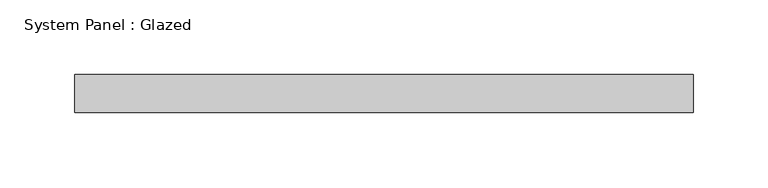
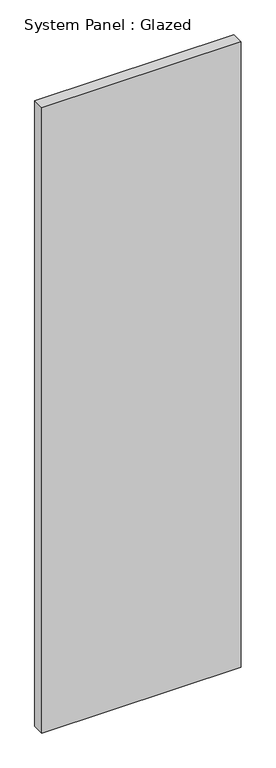
"""IFC4 building model written with IfcOpenShell, lengths in millimetres: plate geometry, System Panel : Glazed."""

from ifc_helpers import new_model, si_unit, origin, origin_with_axes, place, context, project, spatial, polyline, outline, extrude, source, transform, mapped, element, save


def system_panel_glazed_df399847(model_context):
    return source(origin(), model_context, "Body", "SweptSolid", [
        extrude(outline(polyline([(206.375, 19.05), (-206.375, 19.05), (-206.375, 44.45), (206.375, 44.45), (206.375, 19.05)])), origin_with_axes(), (0.0, 0.0, 1.0), 1367.7499719),
    ])


if __name__ == "__main__":
    model = new_model("IFC4")
    model_context = context("Model", 3, world=origin())
    ifc_project = project(units=[si_unit("LENGTHUNIT", "METRE", prefix="MILLI")], contexts=[model_context])
    site = spatial("IfcSite", under=ifc_project)
    building = spatial("IfcBuilding", under=site)
    placement = place(None, origin())
    system_panel_glazed_shape = system_panel_glazed_df399847(model_context)
    element("IfcPlate", 1, ObjectType="System Panel : Glazed", at=placement, inside=building, context=model_context, shape_type="MappedRepresentation", body=[
        mapped(system_panel_glazed_shape, transform((0.0, 0.0, 0.0), x_axis=(1.0, 0.0, 0.0), y_axis=(0.0, 1.0, 0.0), z_axis=(0.0, 0.0, 1.0))),
    ])
    save(model, "model.ifc")

# Revit data of these elements
# Type "System Panel : Glazed"
#   Construction Type Id = "GSP4R"
#   Analytic Construction = "1/8 in Pilkington single glazing"
#   Visual Light Transmittance = 0.9
#   Solar Heat Gain Coefficient = 0.86
#   Heat Transfer Coefficient (U) = 1.18115 BTU/(h·ft²·°F)
#   Define Thermal Properties by = 1
# Element 1 (IfcPlate, "System Panel : Glazed")
#   Materials on its faces: "Glass"
# Materials
#   "Glass": class "Glass", colour RGB 0 128 192, transparency 0.75, Description = "Soda Lime Glass", Cost = 0
